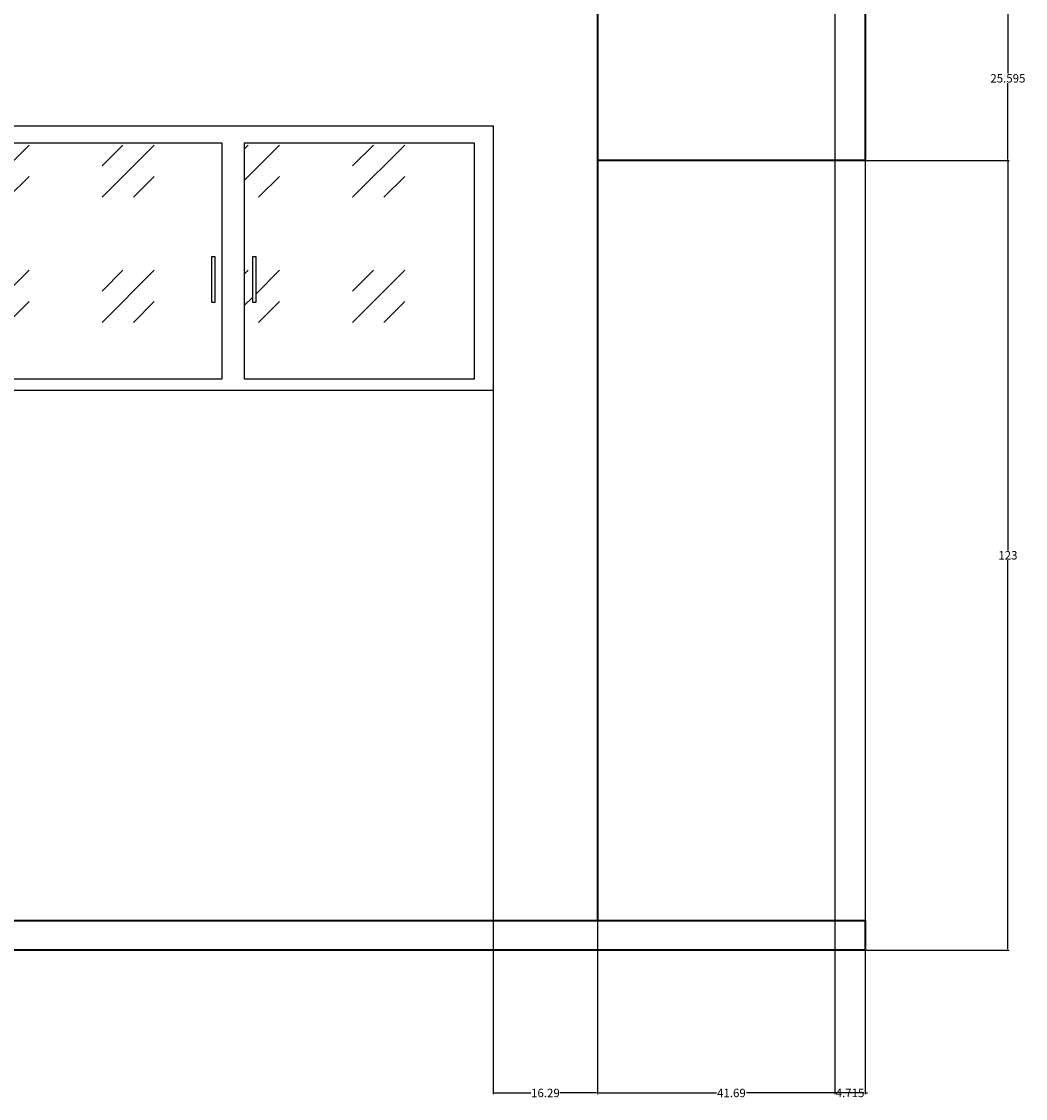
# Model space of a CAD drawing. Units: inches. Extents: x 30 to 515, y 94 to 489.
# Tile 5 of 7: x 358 to 515, y 94 to 262. Entities that reach past the tile are written whole.
import ezdxf

# ---------------------------------------------------------------- set-up
doc = ezdxf.new("R2010")
doc.units = ezdxf.units.IN
doc.header["$MEASUREMENT"] = 0
for name, color, linetype, lineweight in [('A-ANNO-DIMS', 2, 'Continuous', 18), ('A-GLAZ', 4, 'Continuous', 25), ('A-GLAZ-PATT', 8, 'Continuous', 13), ('A-ROOF', 1, 'Continuous', 35), ('A-WALL', 7, 'Continuous', 35)]:
    doc.layers.add(name, color=color, linetype=linetype, lineweight=lineweight)
doc.styles.get("Standard").update_dxf_attribs({"font": 'arial.ttf'})
doc.dimstyles.get("Standard").update_dxf_attribs({"dimtxt": 1.3125, "dimasz": 0.18, "dimexe": 0.18, "dimexo": 0.0625, "dimgap": 0.09, "dimtad": 0, "dimtih": 1, "dimtoh": 1, "dimdec": 4, "dimzin": 0, "dimdsep": 46, "dimlunit": 4, "dimtxsty": 'Standard', "dimcen": 0.09, "dimadec": 0, "dimazin": 0, "dimtfac": 1, "dimtdec": 4, "dimtofl": 0, "dimtmove": 0, "dimatfit": 3, "dimfxl": 1, "dimtolj": 1, "dimtzin": 0, "dimarcsym": 0})

# ---------------------------------------------------------------- blocks, each defined once
blk = doc.blocks.new('WIN-1100-DBL')
for points in [[(0, 41.22), (80.81, 41.22), (80.81, 0), (0, 0)], [(2.73, 38.58), (38.51, 38.58), (38.51, 1.75), (2.73, 1.75)], [(42.07, 38.58), (77.85, 38.58), (77.85, 1.75), (42.07, 1.75)], [(36.99, 20.89), (37.45, 20.89), (37.45, 13.69), (36.99, 13.69)], [(43.35, 20.89), (43.81, 20.89), (43.81, 13.69), (43.35, 13.69)]]:
    blk.add_lwpolyline(points, close=True)
blk = doc.blocks.new('*D13')
at = {"layer": 'A-ANNO-DIMS', "color": 0, "lineweight": -2, "transparency": 16777216}
for p, q in [((448.05, 239.87), (448.05, 94.5)), ((431.76, 204.03), (431.76, 94.5)), ((431.94, 94.68), (437.66, 94.68)), ((447.87, 94.68), (442.15, 94.68))]:
    blk.add_line(p, q, dxfattribs=at)
at = {"layer": 'A-ANNO-DIMS', "color": 0, "transparency": 16777216}
for points in [[(431.94, 94.71), (431.94, 94.65), (431.76, 94.68)], [(447.87, 94.71), (447.87, 94.65), (448.05, 94.68)]]:
    blk.add_solid(points, dxfattribs=at)
at = {"layer": 'Defpoints', "color": 0, "transparency": 16777216}
for p in [(448.05, 239.93), (431.76, 204.09), (448.05, 94.68)]:
    blk.add_point(p, dxfattribs=at)
at = {"layer": 'A-ANNO-DIMS', "color": 0, "transparency": 16777216, "insert": (439.91, 94.68), "char_height": 1.312, "attachment_point": 5}
blk.add_mtext('\\A1;16.29', dxfattribs=at)
blk = doc.blocks.new('*D14')
at = {"layer": 'A-ANNO-DIMS', "color": 0, "lineweight": -2, "transparency": 16777216}
for p, q in [((448.05, 239.87), (448.05, 94.5)), ((489.74, 239.87), (489.74, 94.5)), ((448.23, 94.68), (466.56, 94.68)), ((489.56, 94.68), (471.23, 94.68))]:
    blk.add_line(p, q, dxfattribs=at)
at = {"layer": 'A-ANNO-DIMS', "color": 0, "transparency": 16777216}
for points in [[(448.23, 94.71), (448.23, 94.65), (448.05, 94.68)], [(489.56, 94.71), (489.56, 94.65), (489.74, 94.68)]]:
    blk.add_solid(points, dxfattribs=at)
at = {"layer": 'Defpoints', "color": 0, "transparency": 16777216}
for p in [(448.05, 239.93), (489.74, 239.93), (489.74, 94.68)]:
    blk.add_point(p, dxfattribs=at)
at = {"layer": 'A-ANNO-DIMS', "color": 0, "transparency": 16777216, "insert": (468.9, 94.68), "char_height": 1.312, "attachment_point": 5}
blk.add_mtext('\\A1;41.69', dxfattribs=at)
blk = doc.blocks.new('*D15')
at = {"layer": 'A-ANNO-DIMS', "color": 0, "lineweight": -2, "transparency": 16777216}
for p, q in [((485.027297, 268.465557), (485.027297, 94.504382)), ((489.742649, 265.465557), (489.742649, 94.504382)), ((484.847297, 94.684382), (484.667297, 94.684382)), ((489.922649, 94.684382), (490.102649, 94.684382))]:
    blk.add_line(p, q, dxfattribs=at)
at = {"layer": 'A-ANNO-DIMS', "color": 0, "transparency": 16777216}
for points in [[(484.847297, 94.714382), (484.847297, 94.654382), (485.027297, 94.684382)], [(489.922649, 94.714382), (489.922649, 94.654382), (489.742649, 94.684382)]]:
    blk.add_solid(points, dxfattribs=at)
at = {"layer": 'Defpoints', "color": 0, "transparency": 16777216}
for p in [(485.027297, 268.528057), (489.742649, 265.528057), (489.742649, 94.684382)]:
    blk.add_point(p, dxfattribs=at)
at = {"layer": 'A-ANNO-DIMS', "color": 0, "transparency": 16777216, "insert": (487.384973, 94.684382), "char_height": 1.3125, "attachment_point": 5}
blk.add_mtext('\\A1;4.715', dxfattribs=at)
blk = doc.blocks.new('*D16')
at = {"layer": 'A-ANNO-DIMS', "color": 0, "lineweight": -2, "transparency": 16777216}
for p, q in [((489.81, 239.93), (512.17, 239.93)), ((511.99, 239.75), (511.99, 179.19)), ((511.99, 117.11), (511.99, 177.67)), ((489.81, 116.93), (512.17, 116.93))]:
    blk.add_line(p, q, dxfattribs=at)
at = {"layer": 'A-ANNO-DIMS', "color": 0, "transparency": 16777216}
for points in [[(511.96, 239.75), (512.02, 239.75), (511.99, 239.93)], [(511.96, 117.11), (512.02, 117.11), (511.99, 116.93)]]:
    blk.add_solid(points, dxfattribs=at)
at = {"layer": 'Defpoints', "color": 0, "transparency": 16777216}
for p in [(489.74, 239.93), (511.99, 239.93), (489.74, 116.93)]:
    blk.add_point(p, dxfattribs=at)
at = {"layer": 'A-ANNO-DIMS', "color": 0, "transparency": 16777216, "insert": (511.99, 178.43), "char_height": 1.312, "attachment_point": 5}
blk.add_mtext('\\A1;123', dxfattribs=at)
blk = doc.blocks.new('*D17')
at = {"layer": 'A-ANNO-DIMS', "color": 0, "lineweight": -2, "transparency": 16777216}
for p, q in [((489.81, 265.53), (512.17, 265.53)), ((511.99, 265.35), (511.99, 253.49)), ((511.99, 240.11), (511.99, 251.97)), ((489.81, 239.93), (512.17, 239.93))]:
    blk.add_line(p, q, dxfattribs=at)
at = {"layer": 'A-ANNO-DIMS', "color": 0, "transparency": 16777216}
for points in [[(511.96, 265.35), (512.02, 265.35), (511.99, 265.53)], [(511.96, 240.11), (512.02, 240.11), (511.99, 239.93)]]:
    blk.add_solid(points, dxfattribs=at)
at = {"layer": 'Defpoints', "color": 0, "transparency": 16777216}
for p in [(489.74, 265.53), (511.99, 265.53), (489.74, 239.93)]:
    blk.add_point(p, dxfattribs=at)
at = {"layer": 'A-ANNO-DIMS', "color": 0, "transparency": 16777216, "insert": (511.99, 252.73), "char_height": 1.312, "attachment_point": 5}
blk.add_mtext('\\A1;25.595', dxfattribs=at)

msp = doc.modelspace()

# ---------------------------------------------------------------- hatches: boundary and pattern name
at = {"layer": 'A-GLAZ-PATT'}
h = msp.add_hatch(dxfattribs=at)
h.set_pattern_fill('GOST_GLASS', color=256, scale=2.3)
h.set_pattern_definition([(45, (0, 0), (19.51615, 0), [11.5, -16.1]), (45, (4.879, 0), (19.51615, 0), [4.6, -23]), (45, (0, 4.879), (19.51615, 0), [4.6, -23])])
h.paths.add_polyline_path([(141.7277, 354.4489), (122.2758, 354.4489), (122.2758, 330.4708), (141.7277, 330.4708)])
h.paths.add_polyline_path([(124.1475, 338.9533), (123.2785, 338.9533), (123.2785, 345.0981), (124.1475, 345.0981)], flags=16)
h.paths.add_polyline_path([(120.7384, 354.4489), (101.2865, 354.4489), (101.2865, 330.4708), (120.7384, 330.4708)])
h.paths.add_polyline_path([(119.0673, 338.9533), (119.0673, 345.0981), (119.9363, 345.0981), (119.9363, 338.9533)], flags=16)
h.paths.add_polyline_path([(159.5032, 242.6758), (123.7159, 242.6758), (123.7159, 205.8458), (159.5032, 205.8458)])
h.paths.add_polyline_path([(157.9822, 224.9831), (158.4447, 224.9831), (158.4447, 217.7871), (157.9822, 217.7871)], flags=16)
h.paths.add_polyline_path([(198.8424, 242.6758), (163.0551, 242.6758), (163.0551, 205.8458), (198.8424, 205.8458)])
h.paths.add_polyline_path([(164.8004, 224.9831), (164.8004, 217.7871), (164.3379, 217.7871), (164.3379, 224.9831)], flags=16)
h.paths.add_polyline_path([(389.467, 242.6758), (353.6798, 242.6758), (353.6798, 205.8458), (389.467, 205.8458)])
h.paths.add_polyline_path([(387.946, 224.9831), (388.4085, 224.9831), (388.4085, 217.7871), (387.946, 217.7871)], flags=16)
h.paths.add_polyline_path([(428.8062, 242.6758), (393.0189, 242.6758), (393.0189, 205.8458), (428.8062, 205.8458)])
h.paths.add_polyline_path([(394.7642, 224.9831), (394.7642, 217.7871), (394.3017, 217.7871), (394.3017, 224.9831)], flags=16)

# ---------------------------------------------------------------- linework, layer by layer
at = {"layer": 'A-ROOF'}
for p, q in [((489.7426, 401.4795), (489.7426, 239.9328)), ((489.7426, 239.9328), (448.0511, 239.9328))]:
    msp.add_line(p, q, dxfattribs=at)
at = {"layer": 'A-WALL'}
for p, q in [((448.0511, 265.5281), (448.0511, 121.5281)), ((67.017, 121.5281), (448.0511, 121.5281)), ((448.0511, 121.5281), (489.7426, 121.5281)), ((489.7426, 121.5281), (489.7426, 116.9344)), ((448.0511, 116.9344), (67.017, 116.9344)), ((489.7426, 116.9344), (448.0511, 116.9344))]:
    msp.add_line(p, q, dxfattribs=at)

# ---------------------------------------------------------------- block references
at = {"layer": 'A-GLAZ'}
msp.add_blockref('WIN-1100-DBL', (350.9538, 204.094), dxfattribs=at)

# ---------------------------------------------------------------- dimensions: what is measured, and where the dimension line sits
at = {"layer": 'A-ANNO-DIMS'}
for base, p1, p2, override, picture, middle in [((489.7426, 94.6844), (485.0273, 268.5281), (489.7426, 265.5281), {"dimdec": 3, "dimlfac": 1, "dimrnd": 0, "dimzin": 0, "dimdsep": 46, "dimlunit": 2}, '*D15', (487.385, 94.6844)), ((448.0511, 94.6844), (431.7613, 204.0939), (448.0511, 239.9328), {"dimdec": 2, "dimlfac": 1, "dimrnd": 0, "dimzin": 0, "dimdsep": 46, "dimlunit": 2}, '*D13', (439.9062, 94.6844)), ((489.7426, 94.6844), (448.0511, 239.9328), (489.7426, 239.9328), {"dimdec": 2, "dimlfac": 1, "dimrnd": 0, "dimzin": 0, "dimdsep": 46, "dimlunit": 2}, '*D14', (468.8969, 94.6844))]:
    dim = msp.add_linear_dim(base=base, p1=p1, p2=p2, dimstyle='Standard', override=override, dxfattribs=at)
    dim.commit()
    dim.dimension.update_dxf_attribs({"geometry": picture, "text_midpoint": middle})
for base, p1, p2, override, picture, middle in [((511.9926, 265.5281), (489.7426, 239.9328), (489.7426, 265.5281), {"dimdec": 3, "dimlfac": 1, "dimrnd": 0, "dimzin": 0, "dimdsep": 46, "dimlunit": 2}, '*D17', (511.9926, 252.7304)), ((511.9926, 239.9328), (489.7426, 116.9344), (489.7426, 239.9328), {"dimdec": 0, "dimlfac": 1, "dimrnd": 0, "dimzin": 0, "dimdsep": 46, "dimlunit": 2}, '*D16', (511.9926, 178.4336))]:
    dim = msp.add_linear_dim(base=base, p1=p1, p2=p2, angle=90, dimstyle='Standard', override=override, dxfattribs=at)
    dim.commit()
    dim.dimension.update_dxf_attribs({"geometry": picture, "text_midpoint": middle})

doc.saveas('drawing.dxf')
